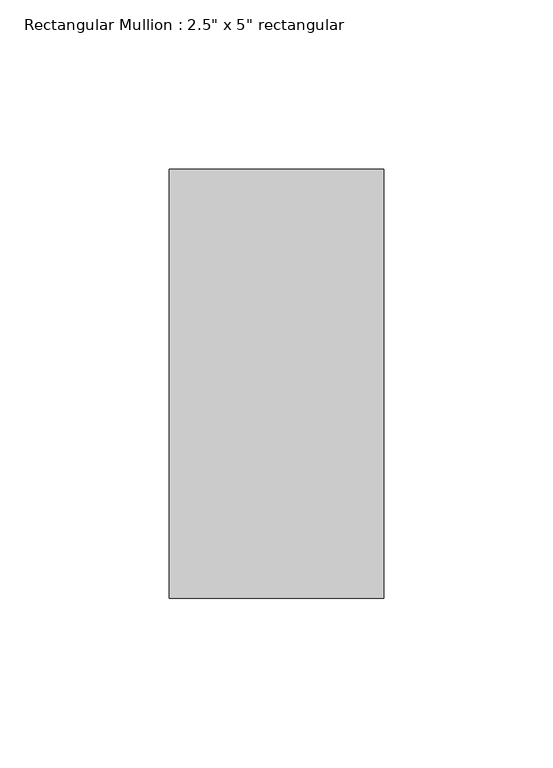
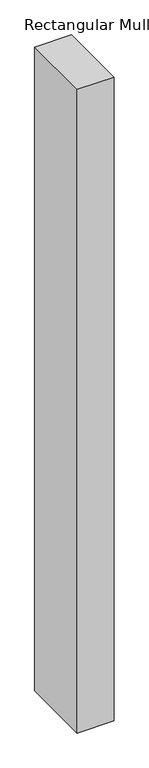
"""IFC4 building model written with IfcOpenShell, lengths in millimetres: member geometry."""

from ifc_helpers import new_model, si_unit, frame, origin, place, context, project, spatial, polyline, outline, extrude, source, transform, mapped, element, save


def member_afffad75(model_context):
    return source(origin(), model_context, "Body", "SweptSolid", [
        extrude(outline(polyline([(31.75, 63.5), (31.75, -63.5), (-31.75, -63.5), (-31.75, 63.5), (31.75, 63.5)])), frame((0.0, 0.0, -1174.2243728), z_axis=(0.0, 0.0, 1.0), x_axis=(1.0, 0.0, 0.0)), (0.0, 0.0, 1.0), 1174.2243728),
    ])


if __name__ == "__main__":
    model = new_model("IFC4")
    model_context = context("Model", 3, world=origin())
    ifc_project = project(units=[si_unit("LENGTHUNIT", "METRE", prefix="MILLI")], contexts=[model_context])
    site = spatial("IfcSite", under=ifc_project)
    building = spatial("IfcBuilding", under=site)
    placement = place(None, origin())
    member_shape = member_afffad75(model_context)
    element("IfcMember", 1, ObjectType="Rectangular Mullion : 2.5\" x 5\" rectangular", at=placement, inside=building, context=model_context, shape_type="MappedRepresentation", body=[
        mapped(member_shape, transform((0.0, 0.0, 0.0), x_axis=(1.0, 0.0, 0.0), y_axis=(0.0, 1.0, 0.0), z_axis=(0.0, 0.0, 1.0))),
    ])
    save(model, "model.ifc")

# Revit data of these elements
# Type "Rectangular Mullion : 2.5\" x 5\" rectangular"
#   built-in parameter 1007304 = 0.416667 (stored number, unit not read)
#   built-in parameter 1007301 = 0.104167 (stored number, unit not read)
#   built-in parameter 1007300 = 0.104167 (stored number, unit not read)
# Element 1 (IfcMember, "Rectangular Mullion : 2.5\" x 5\" rectangular")
#   Materials on its faces: "Aluminum"
# Materials
#   "Aluminum": class "Metal", colour RGB 247 247 247, transparency 0, Description = "Aluminum 6061", Cost = 0
